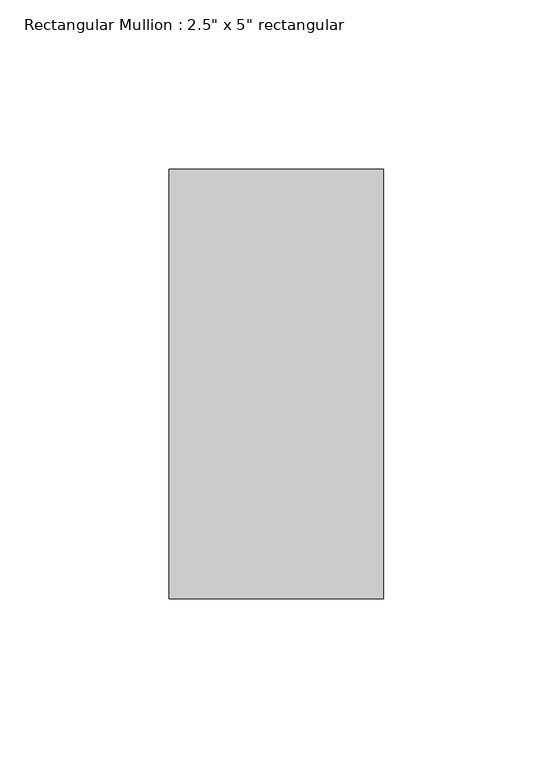
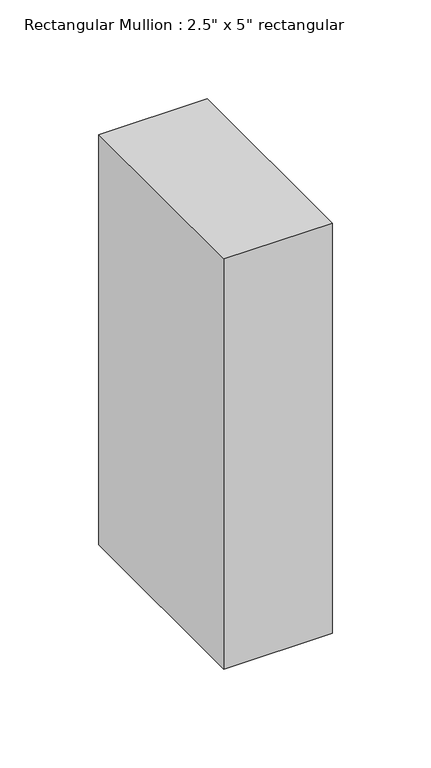
"""IFC4 building model written with IfcOpenShell, lengths in millimetres: member geometry."""

from ifc_helpers import new_model, si_unit, frame, origin, place, context, project, spatial, polyline, outline, extrude, source, transform, mapped, element, save


def member_a44b2684(model_context):
    return source(origin(), model_context, "Body", "SweptSolid", [
        extrude(outline(polyline([(0.0, 63.5), (0.0, -63.5), (-63.5, -63.5), (-63.5, 63.5), (0.0, 63.5)])), frame((0.0, 0.0, -254.0), z_axis=(0.0, 0.0, 1.0), x_axis=(1.0, 0.0, 0.0)), (0.0, 0.0, 1.0), 254.0),
    ])


if __name__ == "__main__":
    model = new_model("IFC4")
    model_context = context("Model", 3, world=origin())
    ifc_project = project(units=[si_unit("LENGTHUNIT", "METRE", prefix="MILLI")], contexts=[model_context])
    site = spatial("IfcSite", under=ifc_project)
    building = spatial("IfcBuilding", under=site)
    placement = place(None, origin())
    member_shape = member_a44b2684(model_context)
    element("IfcMember", 1, ObjectType="Rectangular Mullion : 2.5\" x 5\" rectangular", at=placement, inside=building, context=model_context, shape_type="MappedRepresentation", body=[
        mapped(member_shape, transform((0.0, 0.0, 0.0), x_axis=(1.0, 0.0, 0.0), y_axis=(0.0, 1.0, 0.0), z_axis=(0.0, 0.0, 1.0))),
    ])
    save(model, "model.ifc")

# Revit data of these elements
# Type "Rectangular Mullion : 2.5\" x 5\" rectangular"
#   built-in parameter 1007304 = 0.416667 (stored number, unit not read)
#   built-in parameter 1007301 = 0.104167 (stored number, unit not read)
#   built-in parameter 1007300 = 0.104167 (stored number, unit not read)
# Element 1 (IfcMember, "Rectangular Mullion : 2.5\" x 5\" rectangular")
#   Materials on its faces: "Aluminum"
# Materials
#   "Aluminum": class "Metal", colour RGB 247 247 247, transparency 0, Description = "Aluminum 6061", Cost = 0
